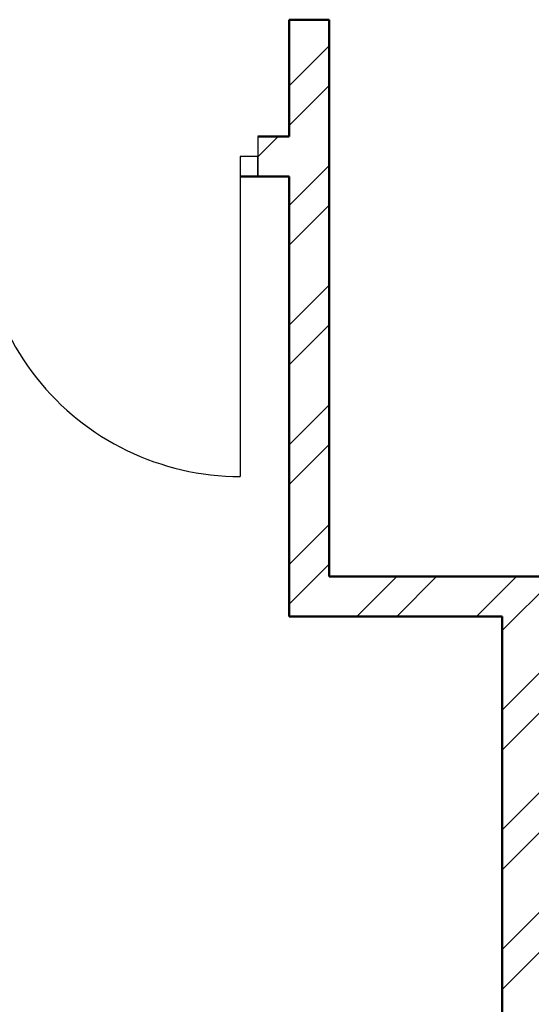
# Model space of a CAD drawing. Units: inches. Extents: x 963 to 2075, y 289 to 2657.
# Tile 67 of 98: x 1342 to 1399, y 2117 to 2228. Entities that reach past the tile are written whole.
import ezdxf

# ---------------------------------------------------------------- set-up
doc = ezdxf.new("R2010")
doc.units = ezdxf.units.IN
for name, color, linetype, lineweight in [('A-DOOR', 4, 'Continuous', 25), ('A-WALL', 7, 'Continuous', 50), ('A-WALL-PATT', 8, 'Continuous', 13)]:
    doc.layers.add(name, color=color, linetype=linetype, lineweight=lineweight)

msp = doc.modelspace()

# ---------------------------------------------------------------- hatches: boundary and pattern name
at = {"layer": 'A-WALL-PATT'}
h = msp.add_hatch(dxfattribs=at)
h.set_pattern_fill('ANSI32', color=256)
h.paths.add_polyline_path([(1473.61, 2163.07), (1473.61, 2165.32), (1376.42, 2165.32), (1376.42, 2227.98), (1371.92, 2227.98), (1371.92, 2214.82), (1368.41, 2214.82), (1368.41, 2210.32), (1371.92, 2210.32), (1371.92, 2160.82), (1395.92, 2160.82), (1395.92, 2090.32), (1217.34, 2090.32), (1217.34, 2085.82), (1395.92, 2085.82), (1458.92, 2085.82), (1458.92, 2108.32), (1454.42, 2108.32), (1454.42, 2090.32), (1400.42, 2090.32), (1400.42, 2160.82), (1473.61, 2160.82)])
h.paths.add_polyline_path([(1649.42, 2210.32), (1653.23, 2210.32), (1653.23, 2214.82), (1649.42, 2214.82), (1649.42, 2227.98), (1644.92, 2227.98), (1644.92, 2165.32), (1550.1, 2165.32), (1550.1, 2160.82), (1620.92, 2160.82), (1620.92, 2112.82), (1555.45, 2112.82), (1555.45, 2108.32), (1584.33, 2108.32), (1584.33, 2084.92), (1588.83, 2084.92), (1588.83, 2108.32), (1625.42, 2108.32), (1667.95, 2108.32), (1667.95, 2022.67), (1588.83, 2022.67), (1588.83, 2047.41), (1584.33, 2047.41), (1584.33, 1996), (1588.83, 1996), (1588.83, 2018.32), (1667.95, 2018.17), (1667.95, 1928.32), (1625.42, 1928.32), (1625.42, 1923.82), (1672.45, 1923.82), (1672.45, 1928.32), (1672.45, 1946.66), (1785.45, 1946.66), (1785.45, 1951.16), (1743.03, 1951.16), (1743.03, 2017.92), (1841.42, 2017.92), (1841.42, 2014.77), (1845.92, 2014.77), (1845.92, 2017.92), (1905.92, 2017.92), (1905.92, 1987.51), (1910.42, 1987.51), (1910.42, 2022.42), (1910.42, 2068.52), (1905.92, 2068.52), (1905.92, 2022.42), (1845.92, 2022.42), (1845.92, 2025.85), (1843.67, 2025.85), (1841.42, 2025.85), (1841.42, 2022.42), (1743.03, 2022.42), (1743.03, 2084.03), (1768.45, 2084.03), (1785.45, 2084.03), (1785.45, 2088.53), (1672.45, 2088.53), (1672.45, 2112.82), (1667.95, 2112.82), (1625.42, 2112.82), (1625.42, 2160.82), (1649.42, 2160.82)])
h.paths.add_polyline_path([(1672.45, 2084.03), (1738.53, 2084.03), (1738.53, 1951.16), (1672.45, 1951.16)], flags=16)
h.paths.add_polyline_path([(1672.45, 2084.03), (1738.53, 2084.03), (1705.49, 2017.6)], flags=0)
h.paths.add_polyline_path([(1262.77, 2085.82), (1258.27, 2085.82), (1258.27, 2023.28), (1184.42, 2023.28), (1184.42, 2018.78), (1258.27, 2018.78), (1258.27, 1950.82), (1262.77, 1950.82)])
h.paths.add_polyline_path([(1312.27, 2085.82), (1307.77, 2085.82), (1307.77, 1950.82), (1312.27, 1950.82)])
h.paths.add_polyline_path([(1458.92, 1950.82), (1395.92, 1950.82), (1216.57, 1950.82), (1216.57, 1946.32), (1346.42, 1946.32), (1395.92, 1946.32), (1395.92, 1875.82), (1371.92, 1875.82), (1371.92, 1826.32), (1368.93, 1826.32), (1368.93, 1821.82), (1371.92, 1821.82), (1371.92, 1813.62), (1376.42, 1813.62), (1376.42, 1871.32), (1474.5, 1871.32), (1474.5, 1873.57), (1474.5, 1875.82), (1400.42, 1875.82), (1400.42, 1946.32), (1454.42, 1946.32), (1454.42, 1928.32), (1458.92, 1928.32)])
h.paths.add_polyline_path([(1184.42, 2120.78), (1167.92, 2120.78), (1167.92, 2134.81), (1165.67, 2134.81), (1163.42, 2134.81), (1163.42, 2120.78), (1119.92, 2120.78), (1119.92, 2098.1), (1124.42, 2098.1), (1124.42, 2116.28), (1167.92, 2116.28), (1179.92, 2116.28), (1179.92, 2045.92), (1184.42, 2045.92), (1184.42, 2090.32), (1184.42, 2116.28)])
h.paths.add_polyline_path([(1124.42, 2018.78), (1179.92, 2018.78), (1179.92, 2016.29), (1184.42, 2016.29), (1184.42, 2023.28), (1184.42, 2026.59), (1182.17, 2026.59), (1179.92, 2026.59), (1179.92, 2023.28), (1124.42, 2023.28), (1124.42, 2074.1), (1119.92, 2074.1), (1119.92, 2018.78), (1119.92, 1979.63), (1124.42, 1979.63)])
h.paths.add_polyline_path([(1184.42, 1925.78), (1184.42, 1946.32), (1184.42, 1996.07), (1182.17, 1996.07), (1179.92, 1996.07), (1179.92, 1925.78), (1124.42, 1925.78), (1124.42, 1955.63), (1119.92, 1955.5), (1119.92, 1921.28), (1158.92, 1921.28), (1158.92, 1909.98), (1163.42, 1909.98), (1163.42, 1921.28), (1184.42, 1921.28)])
h.paths.add_polyline_path([(1341.45, 1826.32), (1163.42, 1826.32), (1163.42, 1849.98), (1158.92, 1849.98), (1158.92, 1821.82), (1158.92, 1804.03), (1163.42, 1804.03), (1163.42, 1821.82), (1341.45, 1821.82)])
h.paths.add_polyline_path([(1222.98, 1713.82), (1163.42, 1713.82), (1163.42, 1744.03), (1161.17, 1744.03), (1158.92, 1744.03), (1158.92, 1713.82), (1119.92, 1713.82), (1119.92, 1694.65), (1124.42, 1694.65), (1124.42, 1709.32), (1158.92, 1709.32), (1222.98, 1709.32)])
h.paths.add_polyline_path([(1328.42, 1713.82), (1252.04, 1713.82), (1252.04, 1711.57), (1252.04, 1709.32), (1256.42, 1709.32), (1256.42, 1547.32), (1232.94, 1547.32), (1232.94, 1545.07), (1232.94, 1542.82), (1292.42, 1542.82), (1292.42, 1527.63), (1296.92, 1527.63), (1296.92, 1542.82), (1299.46, 1542.82), (1299.46, 1547.32), (1260.92, 1547.32), (1260.92, 1658.32), (1343.66, 1658.32), (1343.66, 1660.57), (1343.66, 1662.82), (1328.42, 1662.82), (1328.42, 1676.59), (1327.4, 1676.59), (1323.92, 1676.59), (1323.92, 1662.82), (1260.92, 1662.82), (1260.92, 1709.32), (1323.92, 1709.32), (1323.92, 1699.85), (1328.42, 1699.85)])
h.paths.add_polyline_path([(1649.42, 1875.82), (1625.42, 1875.82), (1625.42, 1928.32), (1620.92, 1928.32), (1588.83, 1928.32), (1588.83, 1950.59), (1584.33, 1950.59), (1584.33, 1928.32), (1555.45, 1928.32), (1555.45, 1923.82), (1620.92, 1923.82), (1620.92, 1875.82), (1548.95, 1875.82), (1548.95, 1873.57), (1548.95, 1871.32), (1644.92, 1871.32), (1644.92, 1813.62), (1649.42, 1813.62), (1649.42, 1821.82), (1652.04, 1821.82), (1652.04, 1824.07), (1652.04, 1826.32), (1649.42, 1826.32)])
h.paths.add_polyline_path([(1512.92, 1871.32), (1516.48, 1871.32), (1516.48, 1875.82), (1512.92, 1875.82), (1512.92, 1923.82), (1512.92, 1928.32), (1512.92, 1930.83), (1508.42, 1930.83), (1508.42, 1875.82), (1504.41, 1875.82), (1504.41, 1871.32), (1508.42, 1871.32), (1508.42, 1713.82), (1376.42, 1713.82), (1376.42, 1743.32), (1371.92, 1743.32), (1371.92, 1709.32), (1371.92, 1706.01), (1376.42, 1706.01), (1376.42, 1709.32), (1508.42, 1709.32), (1508.42, 1547.32), (1501.87, 1547.32), (1501.87, 1542.82), (1508.42, 1542.82), (1508.42, 1482.82), (1508.42, 1436.32), (1512.92, 1436.32), (1512.92, 1542.82), (1519.32, 1542.82), (1519.32, 1545.07), (1519.32, 1547.32), (1512.92, 1547.32), (1512.92, 1709.32), (1644.92, 1709.32), (1644.92, 1707.55), (1649.42, 1707.55), (1649.42, 1709.32), (1649.42, 1743.32), (1644.92, 1743.32), (1644.92, 1713.82), (1512.92, 1713.82)])
h.paths.add_polyline_path([(1129.88, 1545.07), (1129.88, 1547.32), (1124.42, 1547.32), (1095.92, 1547.32), (1095.92, 1614.82), (1124.42, 1614.82), (1124.42, 1619.32), (1095.92, 1619.32), (1091.42, 1619.32), (1091.42, 1542.82), (1095.92, 1542.82), (1119.92, 1542.82), (1129.88, 1542.82)])
h.paths.add_polyline_path([(1208.42, 1542.82), (1211.74, 1542.82), (1211.74, 1547.32), (1198.85, 1547.32), (1198.85, 1542.82), (1203.92, 1542.82), (1203.92, 1478.32), (1208.42, 1478.32), (1296.92, 1478.32), (1296.92, 1503.63), (1292.42, 1503.63), (1292.42, 1482.82), (1208.42, 1482.82)])
h.paths.add_polyline_path([(1430.42, 1542.82), (1435.7, 1542.82), (1435.7, 1545.07), (1435.7, 1547.32), (1422.66, 1547.32), (1422.66, 1545.07), (1422.66, 1542.82), (1425.92, 1542.82), (1425.92, 1482.86), (1341.92, 1482.86), (1341.92, 1502.73), (1337.42, 1502.73), (1337.42, 1478.36), (1425.92, 1478.36), (1425.92, 1440.82), (1425.92, 1436.32), (1430.42, 1436.32)])
h.paths.add_polyline_path([(1698.48, 2004.26), (1727.69, 2004.26), (1727.69, 2022.92), (1698.48, 2022.92)], flags=8)

# ---------------------------------------------------------------- linework, layer by layer
at = {"layer": 'A-DOOR'}
for p, q in [((1368.41, 2214.82), (1368.41, 2210.32)), ((1368.41, 2212.57), (1366.41, 2212.57)), ((1366.41, 2212.57), (1366.41, 2176.57)), ((1368.41, 2210.32), (1368.41, 2212.57))]:
    msp.add_line(p, q, dxfattribs=at)
msp.add_arc((1366.41, 2205.8), 29.23, 166.6115, 270, dxfattribs=at)
at = {"layer": 'A-WALL'}
for p, q in [((1371.92, 2227.98), (1376.42, 2227.98)), ((1371.92, 2227.98), (1371.92, 2214.82)), ((1376.42, 2227.98), (1376.42, 2165.32)), ((1368.41, 2214.82), (1371.92, 2214.82)), ((1366.41, 2210.32), (1371.92, 2210.32)), ((1371.92, 2210.32), (1371.92, 2160.82)), ((1376.42, 2165.32), (1475.02, 2165.32)), ((1371.92, 2160.82), (1395.92, 2160.82)), ((1395.92, 2160.82), (1395.92, 2090.32))]:
    msp.add_line(p, q, dxfattribs=at)

doc.saveas('drawing.dxf')
